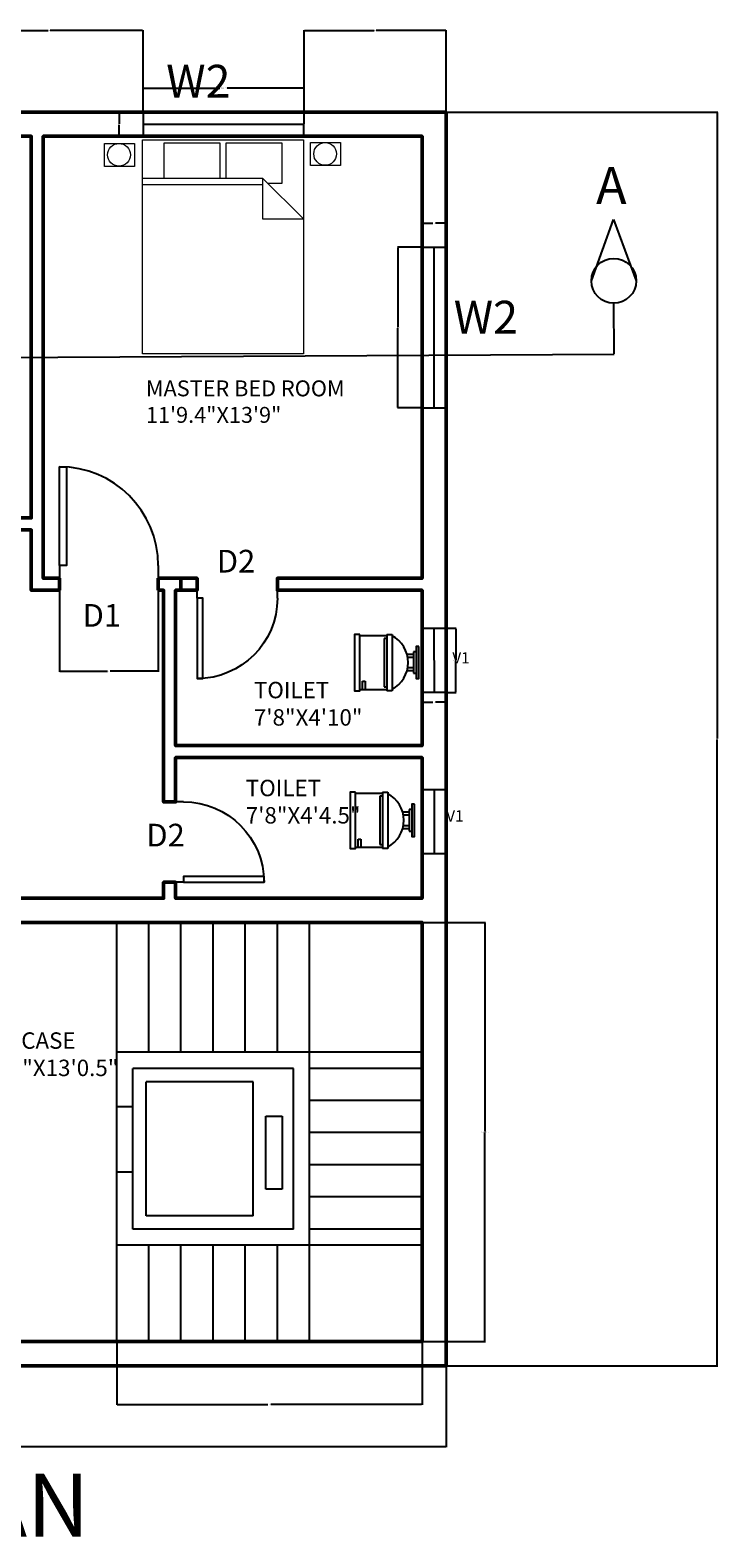
# Model space of a CAD drawing. Units: inches. Extents: x -45 to 1424, y 648 to 1662.
# Tile 3 of 8: x 310 to 567, y 648 to 1211. Entities that reach past the tile are written whole.
import ezdxf

# ---------------------------------------------------------------- set-up
doc = ezdxf.new("R2010")
doc.units = ezdxf.units.IN
for name, color, linetype, lineweight in [('A-ANNO-DIMS', 2, 'Continuous', 18), ('A-ANNO-SYMB', 7, 'Continuous', 25), ('A-ANNO-TEXT', 7, 'Continuous', 18), ('A-ANNO-TITL', 7, 'Continuous', 35), ('A-AREA-IDEN', 7, 'Continuous', 18), ('A-FLOR-EVTR', 140, 'Continuous', 25), ('A-FLOR-FIXT', 3, 'Continuous', 25), ('DOOR', 2, 'Continuous', 25), ('FURNITURE', 3, 'Continuous', 18), ('STAIRCASE', 140, 'Continuous', 25), ('WALL', 4, 'Continuous', 50), ('WINDOW', 1, 'Continuous', 25)]:
    doc.layers.add(name, color=color, linetype=linetype, lineweight=lineweight)
doc.styles.get("Standard").update_dxf_attribs({"font": 'arial.ttf'})
doc.dimstyles.get("Standard").update_dxf_attribs({"dimtxt": 0.18, "dimasz": 0.18, "dimexe": 0.18, "dimexo": 0.0625, "dimgap": 0.09, "dimtad": 0, "dimtih": 1, "dimtoh": 1, "dimdec": 4, "dimzin": 0, "dimdsep": 46, "dimtxsty": 'Standard', "dimcen": 0.09, "dimadec": 0, "dimazin": 0, "dimtfac": 1, "dimtdec": 4, "dimtofl": 0, "dimtmove": 0, "dimatfit": 3, "dimfxl": 1, "dimtolj": 1, "dimtzin": 0, "dimarcsym": 0})

# ---------------------------------------------------------------- blocks, each defined once
blk = doc.blocks.new('*U3')
for p, q in [((0, 0), (0, -6)), ((24, 0), (24, -6))]:
    blk.add_line(p, q)
blk.add_lwpolyline([(0, 0), (0, 24), (1.75, 24), (1.75, 0)], close=True)
blk.add_arc((0, 0), 24, 0, 90)
blk = doc.blocks.new('*U4')
for p, q in [((-24, 0), (-24, 6)), ((0, 0), (0, 6))]:
    blk.add_line(p, q)
blk.add_lwpolyline([(0, 0), (0, -24), (-1.75, -24), (-1.75, 0)], close=True)
blk.add_arc((0, 0), 24, 180, 270)
blk = doc.blocks.new('*U5')
for p, q in [((0, 0), (0, -6)), ((24, 0), (24, -6))]:
    blk.add_line(p, q)
blk.add_lwpolyline([(0, 0), (0, 24), (1.75, 24), (1.75, 0)], close=True)
blk.add_arc((0, 0), 24, 0, 90)
blk = doc.blocks.new('Bed - Queen')
for p, q in [((0, -80.00003), (0, 0)), ((0, 0), (59.99999, 0)), ((59.99999, 0), (59.99999, -80.00003)), ((7.99999, -1.2), (28.79998, -1.2)), ((7.99999, -14.4), (7.99999, -1.2)), ((28.79998, -1.2), (28.79998, -14.4)), ((31.19999, -1.2), (51.99999, -1.2)), ((31.19999, -14.4), (31.19999, -1.2)), ((51.99999, -1.2), (51.99999, -16.4)), ((0, -14.4), (44.8, -14.4)), ((44.8, -16.8), (0, -16.8)), ((59.99999, -29.6), (44.8, -14.4)), ((44.8, -14.4), (44.8, -29.6)), ((51.99999, -16.4), (46.79936, -16.4)), ((44.8, -29.6), (59.99999, -29.6)), ((59.99999, -80.00003), (0, -80.00003))]:
    blk.add_line(p, q)
blk = doc.blocks.new('*U17')
for p, q in [((-254, 558.8), (-254, 304.8)), ((-254, 533.4), (-177.8, 533.4)), ((-177.8, 508), (-254, 508)), ((-177.8, 533.4), (-177.8, 508)), ((254, 304.8), (254, 558.8)), ((266.7, 304.8), (-266.7, 304.8)), ((-266.7, 254), (-266.7, 304.8)), ((228.6, 330.2), (-228.6, 330.2)), ((-228.6, 330.2), (-228.6, 304.8)), ((228.6, 304.8), (228.6, 330.2)), ((266.7, 304.8), (266.7, 254)), ((266.7, 254), (-266.7, 254)), ((101.6, 50.8), (-101.6, 50.8)), ((-101.6, 50.8), (-101.6, 25.4)), ((-76.2, 111.9251), (-76.2, 50.8)), ((-50.8, 50.8), (-50.8, 105.81132)), ((50.8, 105.81132), (50.8, 50.8)), ((76.2, 50.8), (76.2, 111.9251)), ((101.6, 25.4), (101.6, 50.8))]:
    blk.add_line(p, q)
for points in [[(266.7, 558.8), (266.7, 609.6), (-266.7, 609.6), (-266.7, 558.8)], [(152.4, 0), (152.4, 25.4), (-152.4, 25.4), (-152.4, 0)]]:
    blk.add_lwpolyline(points, close=True)
blk.add_arc((0, 389.46582), 287.86658, 208.0725, 331.9275)
blk = doc.blocks.new('WIN-W2-MASTER-N')
for p, q in [((0, 9), (0, 0)), ((60.08, 9), (0, 9)), ((60, 0), (60.08, 9)), ((0, 4.5), (60.04, 4.5)), ((0, 0), (60, 0))]:
    blk.add_line(p, q)
blk = doc.blocks.new('WIN-W2-MASTER-E')
for p, q in [((0, 59.99), (9, 59.99)), ((0, 0), (0, 59.99)), ((4.5, 0), (4.5, 59.99)), ((9, 0), (9, 59.99)), ((0, 0), (9, 0))]:
    blk.add_line(p, q)
blk = doc.blocks.new('VENT-V1-BATH-N')
for p, q in [((0, 24), (9, 24)), ((0, 0), (0, 24)), ((4.65, 0), (4.5, 24)), ((9, 24), (9, 0)), ((9, 0), (0, 0))]:
    blk.add_line(p, q)
blk = doc.blocks.new('VENT-V1-BATH-S')
for p, q in [((0, 24), (9, 24)), ((0, 0), (0, 24)), ((4.5, 24), (4.5, 0)), ((9, 0), (9, 24)), ((9, 0), (0, 0))]:
    blk.add_line(p, q)
blk = doc.blocks.new('FURN-BEDSIDE-UNIT')
blk.add_lwpolyline([(0, 8.55), (11.15, 8.55), (11.15, 0), (0, 0)], close=True)
blk.add_circle((5.42, 4.31), 4.24)
blk = doc.blocks.new('STAIR-RETURN')
for p, q in [((0, 0), (0, 156.5)), ((12, 108), (12, 156.5)), ((24, 108), (24, 156.5)), ((36, 108), (36, 156.5)), ((48, 108), (48, 156.5)), ((60, 108), (60, 156.5)), ((72, 0), (72, 156.5)), ((114, 108), (0, 108)), ((114, 102), (72, 102)), ((114, 90), (72, 90)), ((114, 78), (72, 78)), ((114, 66), (72, 66)), ((114, 66), (72, 66)), ((114, 66), (72, 66)), ((114, 66), (72, 66)), ((114, 54), (72, 54)), ((114, 42), (72, 42)), ((114, 36), (0, 36)), ((12, 0), (12, 36)), ((24, 0), (24, 36)), ((36, 0), (36, 36)), ((48, 0), (48, 36)), ((60, 0), (60, 36))]:
    blk.add_line(p, q)
blk = doc.blocks.new('LIFT-PLAN')
for p, q in [((6, 0), (6, 60)), ((66, 60), (6, 60)), ((66, 0), (66, 60)), ((11, 5), (11, 55)), ((51, 55), (11, 55)), ((51, 5), (51, 55)), ((0, 45.73), (6, 45.73)), ((55.71, 14.94), (55.71, 42.13)), ((55.71, 42.13), (61.81, 42.13)), ((61.81, 42.13), (61.81, 14.94)), ((0, 21.36), (6, 21.36)), ((61.81, 14.94), (55.71, 14.94)), ((51, 5), (11, 5)), ((66, 0), (6, 0))]:
    blk.add_line(p, q)
blk = doc.blocks.new('SECTION-DIRECTION')
for p, q in [((0, 27.32), (8.32, 50.22)), ((8.32, 50.22), (16.73, 27.32)), ((8.52, 0), (8.41, 18.95))]:
    blk.add_line(p, q)
blk.add_circle((8.36, 27.32), 8.36)
blk = doc.blocks.new('*D50')
at = {"layer": 'A-ANNO-DIMS', "color": 0, "lineweight": -2, "transparency": 16777216}
for p, q in [((352.28, 1180.06), (352.28, 1189.19)), ((352.46, 1189.01), (380.97, 1189.01)), ((412.17, 1189.01), (383.66, 1189.01)), ((412.35, 1180.06), (412.35, 1189.19))]:
    blk.add_line(p, q, dxfattribs=at)
at = {"layer": 'A-ANNO-DIMS', "color": 0, "transparency": 16777216}
for points in [[(352.46, 1189.04), (352.46, 1188.98), (352.28, 1189.01)], [(412.17, 1189.04), (412.17, 1188.98), (412.35, 1189.01)]]:
    blk.add_solid(points, dxfattribs=at)
at = {"layer": 'Defpoints', "color": 0, "transparency": 16777216}
for p in [(412.35, 1189.01), (352.28, 1180), (412.35, 1180)]:
    blk.add_point(p, dxfattribs=at)
at = {"layer": 'A-ANNO-DIMS', "color": 0, "transparency": 16777216, "insert": (382.31, 1189.01), "char_height": 0.18, "attachment_point": 5}
blk.add_mtext('\\A1;WINDOW W2 60 TYP.', dxfattribs=at)
blk = doc.blocks.new('*D51')
at = {"layer": 'A-ANNO-DIMS', "color": 0, "lineweight": -2, "transparency": 16777216}
for p, q in [((352.21, 1180), (343.09, 1180)), ((343.27, 1179.82), (343.27, 1175.68)), ((352.21, 1171), (343.09, 1171)), ((343.27, 1171.18), (343.27, 1175.32))]:
    blk.add_line(p, q, dxfattribs=at)
at = {"layer": 'A-ANNO-DIMS', "color": 0, "transparency": 16777216}
for points in [[(343.24, 1179.82), (343.3, 1179.82), (343.27, 1180)], [(343.24, 1171.18), (343.3, 1171.18), (343.27, 1171)]]:
    blk.add_solid(points, dxfattribs=at)
at = {"layer": 'Defpoints', "color": 0, "transparency": 16777216}
for p in [(343.27, 1180), (352.28, 1180), (352.28, 1171)]:
    blk.add_point(p, dxfattribs=at)
at = {"layer": 'A-ANNO-DIMS', "color": 0, "transparency": 16777216, "insert": (343.27, 1175.5), "char_height": 0.18, "attachment_point": 5}
blk.add_mtext('\\A1;9 TYP.', dxfattribs=at)
blk = doc.blocks.new('*D52')
at = {"layer": 'A-ANNO-DIMS', "color": 0, "lineweight": -2, "transparency": 16777216}
for p, q in [((456.34, 1129.56), (447.22, 1129.56)), ((447.4, 1129.38), (447.4, 1099.75)), ((447.4, 1069.75), (447.4, 1099.38)), ((456.34, 1069.57), (447.22, 1069.57))]:
    blk.add_line(p, q, dxfattribs=at)
at = {"layer": 'A-ANNO-DIMS', "color": 0, "transparency": 16777216}
for points in [[(447.37, 1129.38), (447.43, 1129.38), (447.4, 1129.56)], [(447.37, 1069.75), (447.43, 1069.75), (447.4, 1069.57)]]:
    blk.add_solid(points, dxfattribs=at)
at = {"layer": 'Defpoints', "color": 0, "transparency": 16777216}
for p in [(447.4, 1129.56), (456.4, 1129.56), (456.4, 1069.57)]:
    blk.add_point(p, dxfattribs=at)
at = {"layer": 'A-ANNO-DIMS', "color": 0, "transparency": 16777216, "insert": (447.4, 1099.56), "char_height": 0.18, "attachment_point": 5}
blk.add_mtext('\\A1;W2 60 TYP.', dxfattribs=at)
blk = doc.blocks.new('*D53')
at = {"layer": 'A-ANNO-DIMS', "color": 0, "lineweight": -2, "transparency": 16777216}
for p, q in [((456.4, 1129.62), (456.4, 1138.74)), ((456.58, 1138.56), (460.44, 1138.56)), ((465.22, 1138.56), (461.36, 1138.56)), ((465.4, 1129.62), (465.4, 1138.74))]:
    blk.add_line(p, q, dxfattribs=at)
at = {"layer": 'A-ANNO-DIMS', "color": 0, "transparency": 16777216}
for points in [[(456.58, 1138.59), (456.58, 1138.53), (456.4, 1138.56)], [(465.22, 1138.59), (465.22, 1138.53), (465.4, 1138.56)]]:
    blk.add_solid(points, dxfattribs=at)
at = {"layer": 'Defpoints', "color": 0, "transparency": 16777216}
for p in [(465.4, 1138.56), (456.4, 1129.56), (465.4, 1129.56)]:
    blk.add_point(p, dxfattribs=at)
at = {"layer": 'A-ANNO-DIMS', "color": 0, "transparency": 16777216, "insert": (460.9, 1138.56), "char_height": 0.18, "attachment_point": 5}
blk.add_mtext('\\A1;9 TYP.', dxfattribs=at)
blk = doc.blocks.new('*D54')
at = {"layer": 'A-ANNO-DIMS', "color": 0, "lineweight": -2, "transparency": 16777216}
for p, q in [((465.46, 987.3), (469.18, 987.3)), ((469, 987.12), (469, 975.48)), ((469, 963.48), (469, 975.12)), ((465.46, 963.3), (469.18, 963.3))]:
    blk.add_line(p, q, dxfattribs=at)
at = {"layer": 'A-ANNO-DIMS', "color": 0, "transparency": 16777216}
for points in [[(468.97, 987.12), (469.03, 987.12), (469, 987.3)], [(468.97, 963.48), (469.03, 963.48), (469, 963.3)]]:
    blk.add_solid(points, dxfattribs=at)
at = {"layer": 'Defpoints', "color": 0, "transparency": 16777216}
for p in [(465.4, 987.3), (469, 987.3), (465.4, 963.3)]:
    blk.add_point(p, dxfattribs=at)
at = {"layer": 'A-ANNO-DIMS', "color": 0, "transparency": 16777216, "insert": (469, 975.3), "char_height": 0.18, "attachment_point": 5}
blk.add_mtext('\\A1;VENT V1 24 TYP.', dxfattribs=at)
blk = doc.blocks.new('*D55')
at = {"layer": 'A-ANNO-DIMS', "color": 0, "lineweight": -2, "transparency": 16777216}
for p, q in [((456.4, 963.24), (456.4, 959.52)), ((465.4, 963.24), (465.4, 959.52)), ((456.58, 959.7), (460.44, 959.7)), ((465.22, 959.7), (461.36, 959.7))]:
    blk.add_line(p, q, dxfattribs=at)
at = {"layer": 'A-ANNO-DIMS', "color": 0, "transparency": 16777216}
for points in [[(456.58, 959.73), (456.58, 959.67), (456.4, 959.7)], [(465.22, 959.73), (465.22, 959.67), (465.4, 959.7)]]:
    blk.add_solid(points, dxfattribs=at)
at = {"layer": 'Defpoints', "color": 0, "transparency": 16777216}
for p in [(456.4, 963.3), (465.4, 963.3), (465.4, 959.7)]:
    blk.add_point(p, dxfattribs=at)
at = {"layer": 'A-ANNO-DIMS', "color": 0, "transparency": 16777216, "insert": (460.9, 959.7), "char_height": 0.18, "attachment_point": 5}
blk.add_mtext('\\A1;9 TYP.', dxfattribs=at)
blk = doc.blocks.new('*D70')
at = {"layer": 'A-ANNO-DIMS', "color": 0, "lineweight": -2, "transparency": 16777216}
for p, q in [((456.46, 877.5), (480.06, 877.5)), ((479.88, 877.32), (479.88, 799.43)), ((479.88, 721.18), (479.88, 799.07)), ((456.46, 721), (480.06, 721))]:
    blk.add_line(p, q, dxfattribs=at)
at = {"layer": 'A-ANNO-DIMS', "color": 0, "transparency": 16777216}
for points in [[(479.85, 877.32), (479.91, 877.32), (479.88, 877.5)], [(479.85, 721.18), (479.91, 721.18), (479.88, 721)]]:
    blk.add_solid(points, dxfattribs=at)
at = {"layer": 'Defpoints', "color": 0, "transparency": 16777216}
for p in [(456.4, 877.5), (479.88, 877.5), (456.4, 721)]:
    blk.add_point(p, dxfattribs=at)
at = {"layer": 'A-ANNO-DIMS', "color": 0, "transparency": 16777216, "insert": (479.88, 799.25), "char_height": 0.18, "attachment_point": 5}
blk.add_mtext('\\A1;RETURN STAIR 157 TYP.', dxfattribs=at)
blk = doc.blocks.new('*D71')
at = {"layer": 'A-ANNO-DIMS', "color": 0, "lineweight": -2, "transparency": 16777216}
for p, q in [((342.4, 720.94), (342.4, 697.35)), ((456.4, 720.94), (456.4, 697.35)), ((342.58, 697.52), (398.81, 697.52)), ((456.22, 697.52), (399.99, 697.52))]:
    blk.add_line(p, q, dxfattribs=at)
at = {"layer": 'A-ANNO-DIMS', "color": 0, "transparency": 16777216}
for points in [[(342.58, 697.55), (342.58, 697.49), (342.4, 697.52)], [(456.22, 697.55), (456.22, 697.49), (456.4, 697.52)]]:
    blk.add_solid(points, dxfattribs=at)
at = {"layer": 'Defpoints', "color": 0, "transparency": 16777216}
for p in [(342.4, 721), (456.4, 721), (456.4, 697.52)]:
    blk.add_point(p, dxfattribs=at)
at = {"layer": 'A-ANNO-DIMS', "color": 0, "transparency": 16777216, "insert": (399.4, 697.52), "char_height": 0.18, "attachment_point": 5}
blk.add_mtext('\\A1;114 TYP.', dxfattribs=at)
blk = doc.blocks.new('*D74')
at = {"layer": 'A-ANNO-DIMS', "color": 0, "lineweight": -2, "transparency": 16777216}
for p, q in [((40, 711.94), (40, 681.57)), ((465.4, 711.94), (465.4, 681.57)), ((40.18, 681.75), (252.3, 681.75)), ((465.22, 681.75), (253.1, 681.75))]:
    blk.add_line(p, q, dxfattribs=at)
at = {"layer": 'A-ANNO-DIMS', "color": 0, "transparency": 16777216}
for points in [[(40.18, 681.78), (40.18, 681.72), (40, 681.75)], [(465.22, 681.78), (465.22, 681.72), (465.4, 681.75)]]:
    blk.add_solid(points, dxfattribs=at)
at = {"layer": 'Defpoints', "color": 0, "transparency": 16777216}
for p in [(40, 712), (465.4, 712), (465.4, 681.75)]:
    blk.add_point(p, dxfattribs=at)
at = {"layer": 'A-ANNO-DIMS', "color": 0, "transparency": 16777216, "insert": (252.7, 681.75), "char_height": 0.18, "attachment_point": 5}
blk.add_mtext('\\A1;425.4', dxfattribs=at)
blk = doc.blocks.new('*D75')
at = {"layer": 'A-ANNO-DIMS', "color": 0, "lineweight": -2, "transparency": 16777216}
for p, q in [((465.46, 1180), (566.77, 1180)), ((566.59, 1179.82), (566.59, 946.18)), ((566.59, 712.18), (566.59, 945.82)), ((465.46, 712), (566.77, 712))]:
    blk.add_line(p, q, dxfattribs=at)
at = {"layer": 'A-ANNO-DIMS', "color": 0, "transparency": 16777216}
for points in [[(566.56, 1179.82), (566.62, 1179.82), (566.59, 1180)], [(566.56, 712.18), (566.62, 712.18), (566.59, 712)]]:
    blk.add_solid(points, dxfattribs=at)
at = {"layer": 'Defpoints', "color": 0, "transparency": 16777216}
for p in [(465.4, 1180), (566.59, 1180), (465.4, 712)]:
    blk.add_point(p, dxfattribs=at)
at = {"layer": 'A-ANNO-DIMS', "color": 0, "transparency": 16777216, "insert": (566.59, 946), "char_height": 0.18, "attachment_point": 5}
blk.add_mtext('\\A1;468', dxfattribs=at)
blk = doc.blocks.new('*D77')
at = {"layer": 'A-ANNO-DIMS', "color": 0, "lineweight": -2, "transparency": 16777216}
for p, q in [((282.16, 1180.06), (282.16, 1210.61)), ((282.34, 1210.43), (316.83, 1210.43)), ((352.1, 1210.43), (317.61, 1210.43)), ((352.28, 1180.06), (352.28, 1210.61))]:
    blk.add_line(p, q, dxfattribs=at)
at = {"layer": 'A-ANNO-DIMS', "color": 0, "transparency": 16777216}
for points in [[(282.34, 1210.46), (282.34, 1210.4), (282.16, 1210.43)], [(352.1, 1210.46), (352.1, 1210.4), (352.28, 1210.43)]]:
    blk.add_solid(points, dxfattribs=at)
at = {"layer": 'Defpoints', "color": 0, "transparency": 16777216}
for p in [(352.28, 1210.43), (282.16, 1180), (352.28, 1180)]:
    blk.add_point(p, dxfattribs=at)
at = {"layer": 'A-ANNO-DIMS', "color": 0, "transparency": 16777216, "insert": (317.22, 1210.43), "char_height": 0.18, "attachment_point": 5}
blk.add_mtext('\\A1;70.12', dxfattribs=at)
blk = doc.blocks.new('*D78')
at = {"layer": 'A-ANNO-DIMS', "color": 0, "lineweight": -2, "transparency": 16777216}
for p, q in [((412.35, 1180.06), (412.35, 1210.61)), ((412.53, 1210.43), (438.48, 1210.43)), ((465.22, 1210.43), (439.27, 1210.43)), ((465.4, 1180.06), (465.4, 1210.61))]:
    blk.add_line(p, q, dxfattribs=at)
at = {"layer": 'A-ANNO-DIMS', "color": 0, "transparency": 16777216}
for points in [[(412.53, 1210.46), (412.53, 1210.4), (412.35, 1210.43)], [(465.22, 1210.46), (465.22, 1210.4), (465.4, 1210.43)]]:
    blk.add_solid(points, dxfattribs=at)
at = {"layer": 'Defpoints', "color": 0, "transparency": 16777216}
for p in [(465.4, 1210.43), (412.35, 1180), (465.4, 1180)]:
    blk.add_point(p, dxfattribs=at)
at = {"layer": 'A-ANNO-DIMS', "color": 0, "transparency": 16777216, "insert": (438.88, 1210.43), "char_height": 0.18, "attachment_point": 5}
blk.add_mtext('\\A1;53.05', dxfattribs=at)
blk = doc.blocks.new('*D80')
at = {"layer": 'A-ANNO-DIMS', "color": 0, "lineweight": -2, "transparency": 16777216}
for p, q in [((321, 1001.44), (321, 971.07)), ((357.9, 1001.44), (357.9, 971.07)), ((321.18, 971.25), (338.99, 971.25)), ((357.72, 971.25), (339.91, 971.25))]:
    blk.add_line(p, q, dxfattribs=at)
at = {"layer": 'A-ANNO-DIMS', "color": 0, "transparency": 16777216}
for points in [[(321.18, 971.28), (321.18, 971.22), (321, 971.25)], [(357.72, 971.28), (357.72, 971.22), (357.9, 971.25)]]:
    blk.add_solid(points, dxfattribs=at)
at = {"layer": 'Defpoints', "color": 0, "transparency": 16777216}
for p in [(321, 1001.5), (357.9, 1001.5), (321, 971.25)]:
    blk.add_point(p, dxfattribs=at)
at = {"layer": 'A-ANNO-DIMS', "color": 0, "transparency": 16777216, "insert": (339.45, 971.25), "char_height": 0.18, "attachment_point": 5}
blk.add_mtext('\\A1;36.904', dxfattribs=at)

msp = doc.modelspace()

# ---------------------------------------------------------------- linework, layer by layer
at = {"layer": 'A-ANNO-SYMB'}
msp.add_line((-5.8705, 1086.6362), (528.1294, 1089.7026), dxfattribs=at)
at = {"layer": 'WALL'}
for p, q in [((320.997, 1006), (320.997, 1001.5)), ((357.9009, 1006), (357.9009, 1001.5)), ((366.3974, 1001.5), (366.3974, 1006))]:
    msp.add_line(p, q, dxfattribs=at)
msp.add_lwpolyline([(465.4, 1180), (465.4, 712), (40, 712), (40, 1180)], close=True, dxfattribs=at)
for points in [[(320.997, 1001.5), (310.5, 1001.5), (310.5, 1024), (304.5002, 1024), (304.5002, 1028.5), (310.5, 1028.5), (310.5, 1171), (184.5, 1171), (184.5, 1024)], [(357.9009, 1006), (372.3974, 1006), (372.3974, 1001.5), (364.4, 1001.5), (364.4, 943.5), (456.4, 943.5), (456.4, 1001.5), (402.3948, 1001.5), (402.3948, 1006), (456.4, 1006), (456.4, 1171), (315, 1171), (315, 1006), (320.997, 1006)], [(370.3983, 886.5), (456.4, 886.5), (456.4, 939), (364.4, 939), (364.4, 922.4923), (359.9, 922.4923), (359.9, 1001.5), (357.9009, 1001.5)], [(370.3983, 886.5), (364.4, 886.5), (364.4, 892.4923), (359.9, 892.4923), (359.9, 886.5), (270.9, 886.5), (270.9, 854.4), (264.9004, 854.4)], [(279.9, 877.5), (456.4, 877.5), (456.4, 721), (279.9, 721)]]:
    msp.add_lwpolyline(points, dxfattribs=at)

# ---------------------------------------------------------------- block references
at = {"layer": 'A-ANNO-SYMB'}
msp.add_blockref('SECTION-DIRECTION', (519.609, 1089.703), dxfattribs=at)
at = {"layer": 'A-FLOR-EVTR'}
msp.add_blockref('LIFT-PLAN', (342.4, 762.999), dxfattribs=at)
at = {"layer": 'A-FLOR-FIXT', "xscale": 0.0393700787401575, "yscale": 0.0393700787401575, "zscale": 0.0393700787401575, "rotation": 90}
for p in [(455.2031, 974.4977), (453.5882, 915.6044)]:
    msp.add_blockref('*U17', p, dxfattribs=at)
at = {"layer": 'DOOR'}
for name, p, xscale, yscale, zscale in [('*U3', (320.997, 1010.725), 1.537499999999999, 1.537499999999999, 1.537499999999999), ('*U4', (372.3974, 998.5), -1.25, 1.25, 1.25)]:
    msp.add_blockref(name, p, dxfattribs=dict(at, xscale=xscale, yscale=yscale, zscale=zscale))
at = {"layer": 'DOOR', "xscale": -1.25, "yscale": 1.25, "zscale": 1.25, "rotation": 270}
msp.add_blockref('*U5', (367.4, 892.4923), dxfattribs=at)
at = {"layer": 'FURNITURE'}
for name, p in [('FURN-BEDSIDE-UNIT', (337.8516, 1159.7633)), ('Bed - Queen', (352.1005, 1169.7061)), ('FURN-BEDSIDE-UNIT', (414.799, 1160.0884)), ('FURN-BEDSIDE-UNIT', (414.799, 1160.0884))]:
    msp.add_blockref(name, p, dxfattribs=at)
at = {"layer": 'STAIRCASE'}
msp.add_blockref('STAIR-RETURN', (342.4, 721), dxfattribs=at)
at = {"layer": 'WINDOW'}
for name, p in [('WIN-W2-MASTER-N', (352.277, 1171)), ('WIN-W2-MASTER-E', (456.4, 1069.568)), ('VENT-V1-BATH-N', (456.4, 963.301)), ('VENT-V1-BATH-S', (456.4, 903.134))]:
    msp.add_blockref(name, p, dxfattribs=at)

# ---------------------------------------------------------------- texts
at = {"layer": 'A-ANNO-SYMB', "insert": (521.3661, 1159.4625), "char_height": 13.7453, "attachment_point": 1}
msp.add_mtext_dynamic_manual_height_columns('A', width=15.088715, gutter_width=68.7265, heights=[13.7453], dxfattribs=at)
at = {"layer": 'A-ANNO-TEXT', "char_height": 12.26218, "width": 1.05025, "attachment_point": 1}
for insert in [(360.9037, 1197.667), (468.2413, 1109.5826)]:
    msp.add_mtext('W2', dxfattribs=dict(at, insert=insert))
at = {"layer": 'A-ANNO-TEXT', "attachment_point": 1}
for s, width, gutter_width, insert, char_height in [('D2', 4.069942, 42.3777, (379.7709, 1016.587), 8.47554), ('D1', 4.069942, 42.3777, (329.6573, 996.345), 8.47554), ('V1', 24.172645, 21.1047, (467.7052, 978.3762), 4.22094), ('V1', 24.172645, 21.1047, (465.4, 919.3707), 4.22094), ('D2', 4.069942, 42.3777, (353.4701, 914.3115), 8.47554)]:
    msp.add_mtext_dynamic_manual_height_columns(s, width=width, gutter_width=gutter_width, heights=[0], dxfattribs=dict(at, insert=insert, char_height=char_height))
at = {"layer": 'A-ANNO-TITL', "insert": (135.7629, 671.7231), "char_height": 23.5814, "attachment_point": 1}
msp.add_mtext('HOUSE PLAN', dxfattribs=at)
at = {"layer": 'A-AREA-IDEN', "attachment_point": 1}
for s, insert, char_height in [('MASTER BED ROOM\\P11\'9.4"X13\'9"', (353.3237, 1079.8391), 5.93871), ('TOILET\\P7\'8"X4\'10"', (393.6263, 967.2958), 6.1222), ('TOILET\\P7\'8"X4\'4.5"', (390.5952, 930.7361), 6.122202), ('STAIRCASE\\P14\'8.5"X13\'0.5"', (283.9629, 836.4432), 6.122202)]:
    msp.add_mtext(s, dxfattribs=dict(at, insert=insert, char_height=char_height))

# ---------------------------------------------------------------- dimensions: what is measured, and where the dimension line sits
at = {"layer": 'A-ANNO-DIMS'}
for base, p1, p2, override, picture, middle in [((352.2766, 1210.4279), (282.1613, 1180), (352.2766, 1180), {"dimdec": 2, "dimlfac": 1, "dimrnd": 0, "dimzin": 0, "dimdsep": 46, "dimlunit": 2}, '*D77', (317.2189, 1210.4279)), ((465.4, 1210.4279), (412.3525, 1180), (465.4, 1180), {"dimdec": 2, "dimlfac": 1, "dimrnd": 0, "dimzin": 0, "dimdsep": 46, "dimlunit": 2}, '*D78', (438.8763, 1210.4279)), ((465.4, 681.75), (40, 712), (465.4, 712), {"dimdec": 1, "dimlfac": 1, "dimrnd": 0, "dimzin": 0, "dimdsep": 46, "dimlunit": 2}, '*D74', (252.7, 681.75))]:
    dim = msp.add_linear_dim(base=base, p1=p1, p2=p2, dimstyle='Standard', override=override, dxfattribs=at)
    dim.commit()
    dim.dimension.update_dxf_attribs({"geometry": picture, "text_midpoint": middle})
for base, p1, p2, text, picture, middle in [((412.3525, 1189.0114), (352.2766, 1180), (412.3525, 1180), 'WINDOW W2 <> TYP.', '*D50', (382.3146, 1189.0114)), ((465.4, 1138.5575), (456.4, 1129.5588), (465.4, 1129.5588), '<> TYP.', '*D53', (460.9, 1138.5575)), ((465.4, 959.7016), (456.4, 963.3013), (465.4, 963.3013), '<> TYP.', '*D55', (460.9, 959.7016)), ((456.4, 697.525), (342.4, 721), (456.4, 721), '<> TYP.', '*D71', (399.4, 697.525))]:
    dim = msp.add_linear_dim(base=base, p1=p1, p2=p2, text=text, dimstyle='Standard', override={"dimdec": 0, "dimlfac": 1, "dimrnd": 0, "dimzin": 0, "dimdsep": 46, "dimlunit": 2}, dxfattribs=at)
    dim.commit()
    dim.dimension.update_dxf_attribs({"geometry": picture, "text_midpoint": middle})
for base, p1, p2, text, picture, middle in [((343.2652, 1180), (352.2766, 1171), (352.2766, 1180), '<> TYP.', '*D51', (343.2652, 1175.5)), ((447.4014, 1129.5588), (456.4, 1069.5679), (456.4, 1129.5588), 'W2 <> TYP.', '*D52', (447.4014, 1099.5634)), ((468.9997, 987.2996), (465.4, 963.3013), (465.4, 987.2996), 'VENT V1 <> TYP.', '*D54', (468.9997, 975.3004)), ((479.875, 877.5), (456.4, 721), (456.4, 877.5), 'RETURN STAIR <> TYP.', '*D70', (479.875, 799.25))]:
    dim = msp.add_linear_dim(base=base, p1=p1, p2=p2, angle=90, text=text, dimstyle='Standard', override={"dimdec": 0, "dimlfac": 1, "dimrnd": 0, "dimzin": 0, "dimdsep": 46, "dimlunit": 2}, dxfattribs=at)
    dim.commit()
    dim.dimension.update_dxf_attribs({"geometry": picture, "text_midpoint": middle})
for base, p1, p2, angle, override, picture, middle in [((566.5862, 1180), (465.4, 712), (465.4, 1180), 90, {"dimdec": 0, "dimlfac": 1, "dimrnd": 0, "dimzin": 0, "dimdsep": 46, "dimlunit": 2}, '*D75', (566.5862, 946)), ((320.997, 971.25), (357.9009, 1001.5), (320.997, 1001.5), 180, {"dimdec": 3, "dimlfac": 1, "dimrnd": 0, "dimzin": 0, "dimdsep": 46, "dimlunit": 2}, '*D80', (339.4489, 971.25))]:
    dim = msp.add_linear_dim(base=base, p1=p1, p2=p2, angle=angle, dimstyle='Standard', override=override, dxfattribs=at)
    dim.commit()
    dim.dimension.update_dxf_attribs({"geometry": picture, "text_midpoint": middle})

doc.saveas('drawing.dxf')
